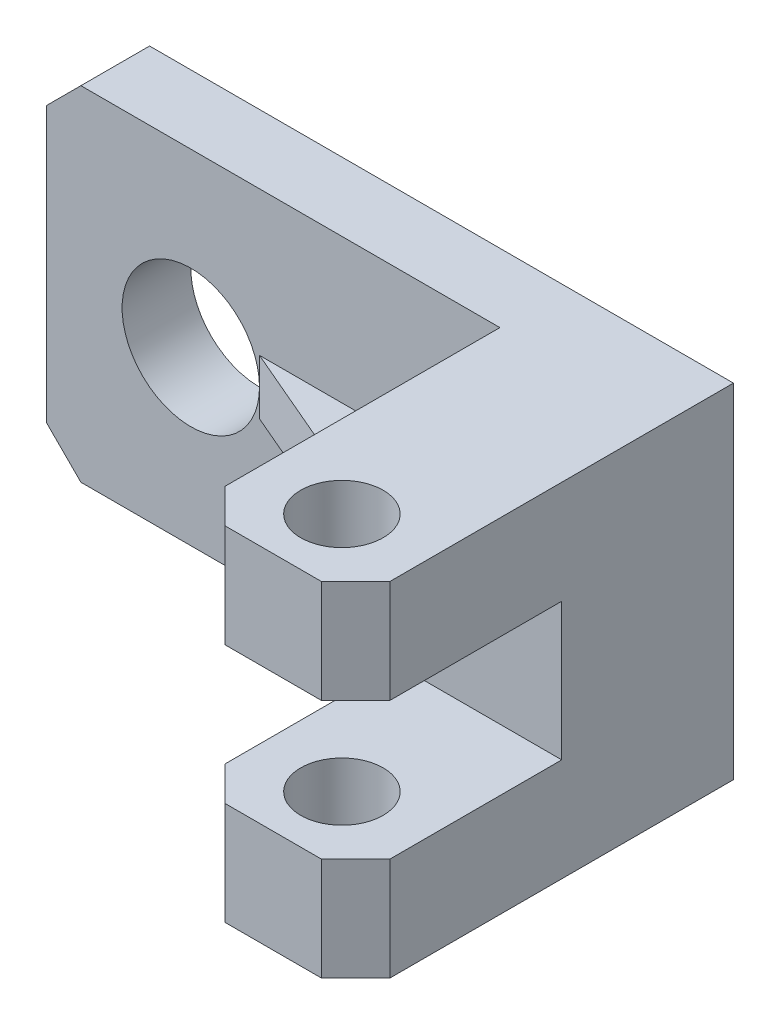
ISO-10303-21;
HEADER;
FILE_DESCRIPTION(('STEP AP214'),'2;1');
FILE_NAME('part.step','',(''),(''),'','','');
FILE_SCHEMA(('AUTOMOTIVE_DESIGN { 1 0 10303 214 1 1 1 1 }'));
ENDSEC;
DATA;
#1=APPLICATION_CONTEXT('core data for automotive mechanical design processes');
#2=APPLICATION_PROTOCOL_DEFINITION('international standard','automotive_design',2000,#1);
#3=PRODUCT_CONTEXT('',#1,'mechanical');
#4=PRODUCT('Part','Part','',(#3));
#5=PRODUCT_RELATED_PRODUCT_CATEGORY('part','',(#4));
#6=PRODUCT_DEFINITION_FORMATION('','',#4);
#7=PRODUCT_DEFINITION_CONTEXT('part definition',#1,'design');
#8=PRODUCT_DEFINITION('design','',#6,#7);
#9=PRODUCT_DEFINITION_SHAPE('','',#8);
#10=(LENGTH_UNIT() NAMED_UNIT(*) SI_UNIT(.MILLI.,.METRE.));
#11=(NAMED_UNIT(*) PLANE_ANGLE_UNIT() SI_UNIT($,.RADIAN.));
#12=(NAMED_UNIT(*) SI_UNIT($,.STERADIAN.) SOLID_ANGLE_UNIT());
#13=UNCERTAINTY_MEASURE_WITH_UNIT(LENGTH_MEASURE(1.E-05),#10,'distance_accuracy_value','');
#14=(GEOMETRIC_REPRESENTATION_CONTEXT(3) GLOBAL_UNCERTAINTY_ASSIGNED_CONTEXT((#13)) GLOBAL_UNIT_ASSIGNED_CONTEXT((#10,
#11,#12)) REPRESENTATION_CONTEXT('',''));
#15=CARTESIAN_POINT('',(0.,0.,0.));
#16=DIRECTION('',(0.,0.,1.));
#17=DIRECTION('',(1.,0.,0.));
#18=AXIS2_PLACEMENT_3D('',#15,#16,#17);
#19=CARTESIAN_POINT('',(66.,50.,50.));
#20=DIRECTION('',(-1.,0.,0.));
#21=DIRECTION('',(0.,0.,1.));
#22=AXIS2_PLACEMENT_3D('',#19,#20,#21);
#23=PLANE('',#22);
#24=DIRECTION('',(0.,-1.,0.));
#25=VECTOR('',#24,1.);
#26=CARTESIAN_POINT('',(66.,15.,25.));
#27=LINE('',#26,#25);
#28=CARTESIAN_POINT('',(66.,35.,25.));
#29=VERTEX_POINT('',#28);
#30=CARTESIAN_POINT('',(66.,29.,25.));
#31=VERTEX_POINT('',#30);
#32=EDGE_CURVE('E198',#29,#31,#27,.T.);
#33=ORIENTED_EDGE('',*,*,#32,.F.);
#34=DIRECTION('',(0.,0.,1.));
#35=VECTOR('',#34,1.);
#36=CARTESIAN_POINT('',(66.,35.,30.));
#37=LINE('',#36,#35);
#38=CARTESIAN_POINT('',(66.,35.,50.));
#39=VERTEX_POINT('',#38);
#40=EDGE_CURVE('E182',#29,#39,#37,.T.);
#41=ORIENTED_EDGE('',*,*,#40,.T.);
#42=DIRECTION('',(0.,-1.,0.));
#43=VECTOR('',#42,1.);
#44=CARTESIAN_POINT('',(66.,50.,50.));
#45=LINE('',#44,#43);
#46=CARTESIAN_POINT('',(66.,50.,50.));
#47=VERTEX_POINT('',#46);
#48=EDGE_CURVE('E290',#47,#39,#45,.T.);
#49=ORIENTED_EDGE('',*,*,#48,.F.);
#50=DIRECTION('',(0.,0.,-1.));
#51=VECTOR('',#50,1.);
#52=CARTESIAN_POINT('',(66.,50.,50.));
#53=LINE('',#52,#51);
#54=CARTESIAN_POINT('',(66.,50.,10.));
#55=VERTEX_POINT('',#54);
#56=EDGE_CURVE('E277',#47,#55,#53,.T.);
#57=ORIENTED_EDGE('',*,*,#56,.T.);
#58=DIRECTION('',(0.,1.,0.));
#59=VECTOR('',#58,1.);
#60=CARTESIAN_POINT('',(66.,29.,10.));
#61=LINE('',#60,#59);
#62=CARTESIAN_POINT('',(66.,29.,10.));
#63=VERTEX_POINT('',#62);
#64=EDGE_CURVE('E217',#63,#55,#61,.T.);
#65=ORIENTED_EDGE('',*,*,#64,.F.);
#66=DIRECTION('',(0.,0.,-1.));
#67=VECTOR('',#66,1.);
#68=CARTESIAN_POINT('',(66.,29.,25.));
#69=LINE('',#68,#67);
#70=EDGE_CURVE('E207',#31,#63,#69,.T.);
#71=ORIENTED_EDGE('',*,*,#70,.F.);
#72=EDGE_LOOP('',(#33,#41,#49,#57,#65,#71));
#73=FACE_BOUND('',#72,.T.);
#74=ADVANCED_FACE('F44',(#73),#23,.T.);
#75=CARTESIAN_POINT('',(31.,50.,10.));
#76=DIRECTION('',(-0.393919298579168,0.,0.919145030018058));
#77=DIRECTION('',(0.919145030018058,0.,0.393919298579168));
#78=AXIS2_PLACEMENT_3D('',#75,#76,#77);
#79=PLANE('',#78);
#80=DIRECTION('',(0.,-1.,0.));
#81=VECTOR('',#80,1.);
#82=CARTESIAN_POINT('',(66.,50.,25.));
#83=LINE('',#82,#81);
#84=CARTESIAN_POINT('',(66.,21.,25.));
#85=VERTEX_POINT('',#84);
#86=EDGE_CURVE('E235',#31,#85,#83,.T.);
#87=ORIENTED_EDGE('',*,*,#86,.F.);
#88=DIRECTION('',(0.919145030018058,0.,0.393919298579168));
#89=VECTOR('',#88,1.);
#90=CARTESIAN_POINT('',(31.,29.,10.));
#91=LINE('',#90,#89);
#92=CARTESIAN_POINT('',(31.,29.,10.));
#93=VERTEX_POINT('',#92);
#94=EDGE_CURVE('E214',#93,#31,#91,.T.);
#95=ORIENTED_EDGE('',*,*,#94,.F.);
#96=DIRECTION('',(0.,-1.,0.));
#97=VECTOR('',#96,1.);
#98=CARTESIAN_POINT('',(31.,50.,10.));
#99=LINE('',#98,#97);
#100=CARTESIAN_POINT('',(31.,25.,10.));
#101=VERTEX_POINT('',#100);
#102=EDGE_CURVE('E231',#93,#101,#99,.T.);
#103=ORIENTED_EDGE('',*,*,#102,.T.);
#104=CARTESIAN_POINT('',(31.,21.,10.));
#105=VERTEX_POINT('',#104);
#106=EDGE_CURVE('E236',#101,#105,#99,.T.);
#107=ORIENTED_EDGE('',*,*,#106,.T.);
#108=DIRECTION('',(-0.919145030018058,0.,-0.393919298579168));
#109=VECTOR('',#108,1.);
#110=CARTESIAN_POINT('',(31.,21.,10.));
#111=LINE('',#110,#109);
#112=EDGE_CURVE('E220',#85,#105,#111,.T.);
#113=ORIENTED_EDGE('',*,*,#112,.F.);
#114=EDGE_LOOP('',(#87,#95,#103,#107,#113));
#115=FACE_BOUND('',#114,.T.);
#116=ADVANCED_FACE('F365',(#115),#79,.T.);
#117=CARTESIAN_POINT('',(71.,50.,55.));
#118=DIRECTION('',(-0.707106781186547,0.,0.707106781186548));
#119=DIRECTION('',(0.707106781186548,0.,0.707106781186547));
#120=AXIS2_PLACEMENT_3D('',#117,#118,#119);
#121=PLANE('',#120);
#122=DIRECTION('',(-0.707106781186548,0.,-0.707106781186547));
#123=VECTOR('',#122,1.);
#124=CARTESIAN_POINT('',(71.,35.,55.));
#125=LINE('',#124,#123);
#126=CARTESIAN_POINT('',(71.,35.,55.));
#127=VERTEX_POINT('',#126);
#128=EDGE_CURVE('E188',#127,#39,#125,.T.);
#129=ORIENTED_EDGE('',*,*,#128,.F.);
#130=DIRECTION('',(0.,-1.,0.));
#131=VECTOR('',#130,1.);
#132=CARTESIAN_POINT('',(71.,50.,55.));
#133=LINE('',#132,#131);
#134=CARTESIAN_POINT('',(71.,50.,55.));
#135=VERTEX_POINT('',#134);
#136=EDGE_CURVE('E291',#135,#127,#133,.T.);
#137=ORIENTED_EDGE('',*,*,#136,.F.);
#138=DIRECTION('',(-0.707106781186548,0.,-0.707106781186547));
#139=VECTOR('',#138,1.);
#140=CARTESIAN_POINT('',(71.,50.,55.));
#141=LINE('',#140,#139);
#142=EDGE_CURVE('E271',#135,#47,#141,.T.);
#143=ORIENTED_EDGE('',*,*,#142,.T.);
#144=ORIENTED_EDGE('',*,*,#48,.T.);
#145=EDGE_LOOP('',(#129,#137,#143,#144));
#146=FACE_BOUND('',#145,.T.);
#147=ADVANCED_FACE('F368',(#146),#121,.T.);
#148=CARTESIAN_POINT('',(71.,50.,55.));
#149=DIRECTION('',(0.,0.,1.));
#150=DIRECTION('',(1.,0.,0.));
#151=AXIS2_PLACEMENT_3D('',#148,#149,#150);
#152=PLANE('',#151);
#153=DIRECTION('',(-1.,0.,0.));
#154=VECTOR('',#153,1.);
#155=CARTESIAN_POINT('',(66.,35.,55.));
#156=LINE('',#155,#154);
#157=CARTESIAN_POINT('',(85.,35.,55.));
#158=VERTEX_POINT('',#157);
#159=EDGE_CURVE('E242',#158,#127,#156,.T.);
#160=ORIENTED_EDGE('',*,*,#159,.F.);
#161=DIRECTION('',(0.,-1.,0.));
#162=VECTOR('',#161,1.);
#163=CARTESIAN_POINT('',(85.,50.,55.));
#164=LINE('',#163,#162);
#165=CARTESIAN_POINT('',(85.,50.,55.));
#166=VERTEX_POINT('',#165);
#167=EDGE_CURVE('E300',#166,#158,#164,.T.);
#168=ORIENTED_EDGE('',*,*,#167,.F.);
#169=DIRECTION('',(-1.,0.,0.));
#170=VECTOR('',#169,1.);
#171=CARTESIAN_POINT('',(71.,50.,55.));
#172=LINE('',#171,#170);
#173=EDGE_CURVE('E270',#166,#135,#172,.T.);
#174=ORIENTED_EDGE('',*,*,#173,.T.);
#175=ORIENTED_EDGE('',*,*,#136,.T.);
#176=EDGE_LOOP('',(#160,#168,#174,#175));
#177=FACE_BOUND('',#176,.T.);
#178=ADVANCED_FACE('F428',(#177),#152,.T.);
#179=CARTESIAN_POINT('',(85.,50.,55.));
#180=DIRECTION('',(0.707106781186547,0.,0.707106781186548));
#181=DIRECTION('',(0.707106781186548,0.,-0.707106781186547));
#182=AXIS2_PLACEMENT_3D('',#179,#180,#181);
#183=PLANE('',#182);
#184=DIRECTION('',(-0.707106781186548,0.,0.707106781186547));
#185=VECTOR('',#184,1.);
#186=CARTESIAN_POINT('',(85.,35.,55.));
#187=LINE('',#186,#185);
#188=CARTESIAN_POINT('',(90.,35.,50.));
#189=VERTEX_POINT('',#188);
#190=EDGE_CURVE('E257',#189,#158,#187,.T.);
#191=ORIENTED_EDGE('',*,*,#190,.F.);
#192=DIRECTION('',(0.,-1.,0.));
#193=VECTOR('',#192,1.);
#194=CARTESIAN_POINT('',(90.,50.,50.));
#195=LINE('',#194,#193);
#196=CARTESIAN_POINT('',(90.,50.,50.));
#197=VERTEX_POINT('',#196);
#198=EDGE_CURVE('E301',#197,#189,#195,.T.);
#199=ORIENTED_EDGE('',*,*,#198,.F.);
#200=DIRECTION('',(-0.707106781186548,0.,0.707106781186547));
#201=VECTOR('',#200,1.);
#202=CARTESIAN_POINT('',(85.,50.,55.));
#203=LINE('',#202,#201);
#204=EDGE_CURVE('E268',#197,#166,#203,.T.);
#205=ORIENTED_EDGE('',*,*,#204,.T.);
#206=ORIENTED_EDGE('',*,*,#167,.T.);
#207=EDGE_LOOP('',(#191,#199,#205,#206));
#208=FACE_BOUND('',#207,.T.);
#209=ADVANCED_FACE('F429',(#208),#183,.T.);
#210=CARTESIAN_POINT('',(78.,50.,45.));
#211=DIRECTION('',(0.,-1.,0.));
#212=DIRECTION('',(0.,0.,-1.));
#213=AXIS2_PLACEMENT_3D('',#210,#211,#212);
#214=CYLINDRICAL_SURFACE('',#213,6.);
#215=CARTESIAN_POINT('',(78.,35.,45.));
#216=DIRECTION('',(0.,1.,0.));
#217=DIRECTION('',(0.,0.,1.));
#218=AXIS2_PLACEMENT_3D('',#215,#216,#217);
#219=CIRCLE('',#218,6.);
#220=CARTESIAN_POINT('',(78.,35.,51.));
#221=VERTEX_POINT('',#220);
#222=EDGE_CURVE('E47',#221,#221,#219,.F.);
#223=ORIENTED_EDGE('',*,*,#222,.T.);
#224=EDGE_LOOP('',(#223));
#225=FACE_BOUND('',#224,.T.);
#226=CARTESIAN_POINT('',(78.,50.,45.));
#227=DIRECTION('',(0.,-1.,0.));
#228=DIRECTION('',(0.,0.,-1.));
#229=AXIS2_PLACEMENT_3D('',#226,#227,#228);
#230=CIRCLE('',#229,6.);
#231=CARTESIAN_POINT('',(78.,50.,39.));
#232=VERTEX_POINT('',#231);
#233=EDGE_CURVE('E258',#232,#232,#230,.T.);
#234=ORIENTED_EDGE('',*,*,#233,.F.);
#235=EDGE_LOOP('',(#234));
#236=FACE_BOUND('',#235,.T.);
#237=ADVANCED_FACE('F435',(#225,#236),#214,.F.);
#238=CARTESIAN_POINT('',(0.,0.,10.));
#239=DIRECTION('',(0.,0.,-1.));
#240=DIRECTION('',(-1.,0.,0.));
#241=AXIS2_PLACEMENT_3D('',#238,#239,#240);
#242=PLANE('',#241);
#243=DIRECTION('',(1.,0.,0.));
#244=VECTOR('',#243,1.);
#245=CARTESIAN_POINT('',(90.,0.,10.));
#246=LINE('',#245,#244);
#247=CARTESIAN_POINT('',(4.99999999999999,0.,10.));
#248=VERTEX_POINT('',#247);
#249=CARTESIAN_POINT('',(66.,0.,10.));
#250=VERTEX_POINT('',#249);
#251=EDGE_CURVE('E315',#248,#250,#246,.T.);
#252=ORIENTED_EDGE('',*,*,#251,.T.);
#253=DIRECTION('',(0.,-1.,0.));
#254=VECTOR('',#253,1.);
#255=CARTESIAN_POINT('',(66.,21.,10.));
#256=LINE('',#255,#254);
#257=CARTESIAN_POINT('',(66.,21.,10.));
#258=VERTEX_POINT('',#257);
#259=EDGE_CURVE('E230',#258,#250,#256,.T.);
#260=ORIENTED_EDGE('',*,*,#259,.F.);
#261=DIRECTION('',(1.,0.,0.));
#262=VECTOR('',#261,1.);
#263=CARTESIAN_POINT('',(66.,21.,10.));
#264=LINE('',#263,#262);
#265=EDGE_CURVE('E222',#105,#258,#264,.T.);
#266=ORIENTED_EDGE('',*,*,#265,.F.);
#267=ORIENTED_EDGE('',*,*,#106,.F.);
#268=CARTESIAN_POINT('',(21.,25.,10.));
#269=DIRECTION('',(0.,0.,1.));
#270=DIRECTION('',(1.,0.,0.));
#271=AXIS2_PLACEMENT_3D('',#268,#269,#270);
#272=CIRCLE('',#271,9.99999999999999);
#273=EDGE_CURVE('E232',#101,#101,#272,.T.);
#274=ORIENTED_EDGE('',*,*,#273,.F.);
#275=ORIENTED_EDGE('',*,*,#102,.F.);
#276=DIRECTION('',(-1.,0.,0.));
#277=VECTOR('',#276,1.);
#278=CARTESIAN_POINT('',(66.,29.,10.));
#279=LINE('',#278,#277);
#280=EDGE_CURVE('E65',#63,#93,#279,.T.);
#281=ORIENTED_EDGE('',*,*,#280,.F.);
#282=ORIENTED_EDGE('',*,*,#64,.T.);
#283=DIRECTION('',(-1.,0.,0.));
#284=VECTOR('',#283,1.);
#285=CARTESIAN_POINT('',(90.,50.,10.));
#286=LINE('',#285,#284);
#287=CARTESIAN_POINT('',(4.99999999999999,50.,10.));
#288=VERTEX_POINT('',#287);
#289=EDGE_CURVE('E314',#55,#288,#286,.T.);
#290=ORIENTED_EDGE('',*,*,#289,.T.);
#291=DIRECTION('',(-0.707106781186547,-0.707106781186548,0.));
#292=VECTOR('',#291,1.);
#293=CARTESIAN_POINT('',(0.,45.,10.));
#294=LINE('',#293,#292);
#295=CARTESIAN_POINT('',(0.,45.,10.));
#296=VERTEX_POINT('',#295);
#297=EDGE_CURVE('E302',#288,#296,#294,.T.);
#298=ORIENTED_EDGE('',*,*,#297,.T.);
#299=DIRECTION('',(0.,-1.,0.));
#300=VECTOR('',#299,1.);
#301=CARTESIAN_POINT('',(0.,45.,10.));
#302=LINE('',#301,#300);
#303=CARTESIAN_POINT('',(0.,5.,10.));
#304=VERTEX_POINT('',#303);
#305=EDGE_CURVE('E310',#296,#304,#302,.T.);
#306=ORIENTED_EDGE('',*,*,#305,.T.);
#307=DIRECTION('',(0.707106781186546,-0.707106781186548,0.));
#308=VECTOR('',#307,1.);
#309=CARTESIAN_POINT('',(0.,5.,10.));
#310=LINE('',#309,#308);
#311=EDGE_CURVE('E309',#304,#248,#310,.T.);
#312=ORIENTED_EDGE('',*,*,#311,.T.);
#313=EDGE_LOOP('',(#252,#260,#266,#267,#274,#275,#281,#282,#290,#298,#306,#312));
#314=FACE_BOUND('',#313,.T.);
#315=ADVANCED_FACE('F417',(#314),#242,.F.);
#316=CARTESIAN_POINT('',(0.,45.,10.));
#317=DIRECTION('',(0.707106781186548,-0.707106781186547,0.));
#318=DIRECTION('',(0.707106781186547,0.707106781186548,0.));
#319=AXIS2_PLACEMENT_3D('',#316,#317,#318);
#320=PLANE('',#319);
#321=DIRECTION('',(-0.707106781186547,-0.707106781186548,0.));
#322=VECTOR('',#321,1.);
#323=CARTESIAN_POINT('',(0.,45.,0.));
#324=LINE('',#323,#322);
#325=CARTESIAN_POINT('',(4.99999999999999,50.,0.));
#326=VERTEX_POINT('',#325);
#327=CARTESIAN_POINT('',(0.,45.,0.));
#328=VERTEX_POINT('',#327);
#329=EDGE_CURVE('E293',#326,#328,#324,.T.);
#330=ORIENTED_EDGE('',*,*,#329,.T.);
#331=DIRECTION('',(0.,0.,-1.));
#332=VECTOR('',#331,1.);
#333=CARTESIAN_POINT('',(0.,45.,10.));
#334=LINE('',#333,#332);
#335=EDGE_CURVE('E11',#296,#328,#334,.T.);
#336=ORIENTED_EDGE('',*,*,#335,.F.);
#337=ORIENTED_EDGE('',*,*,#297,.F.);
#338=DIRECTION('',(0.,0.,-1.));
#339=VECTOR('',#338,1.);
#340=CARTESIAN_POINT('',(4.99999999999999,50.,10.));
#341=LINE('',#340,#339);
#342=EDGE_CURVE('E320',#288,#326,#341,.T.);
#343=ORIENTED_EDGE('',*,*,#342,.T.);
#344=EDGE_LOOP('',(#330,#336,#337,#343));
#345=FACE_BOUND('',#344,.T.);
#346=ADVANCED_FACE('F50',(#345),#320,.F.);
#347=CARTESIAN_POINT('',(0.,45.,10.));
#348=DIRECTION('',(1.,0.,0.));
#349=DIRECTION('',(0.,0.,-1.));
#350=AXIS2_PLACEMENT_3D('',#347,#348,#349);
#351=PLANE('',#350);
#352=DIRECTION('',(0.,-1.,0.));
#353=VECTOR('',#352,1.);
#354=CARTESIAN_POINT('',(0.,45.,0.));
#355=LINE('',#354,#353);
#356=CARTESIAN_POINT('',(0.,5.,0.));
#357=VERTEX_POINT('',#356);
#358=EDGE_CURVE('E318',#328,#357,#355,.T.);
#359=ORIENTED_EDGE('',*,*,#358,.T.);
#360=DIRECTION('',(0.,0.,-1.));
#361=VECTOR('',#360,1.);
#362=CARTESIAN_POINT('',(0.,5.,10.));
#363=LINE('',#362,#361);
#364=EDGE_CURVE('E53',#304,#357,#363,.T.);
#365=ORIENTED_EDGE('',*,*,#364,.F.);
#366=ORIENTED_EDGE('',*,*,#305,.F.);
#367=ORIENTED_EDGE('',*,*,#335,.T.);
#368=EDGE_LOOP('',(#359,#365,#366,#367));
#369=FACE_BOUND('',#368,.T.);
#370=ADVANCED_FACE('F532',(#369),#351,.F.);
#371=CARTESIAN_POINT('',(0.,5.,10.));
#372=DIRECTION('',(0.707106781186548,0.707106781186546,0.));
#373=DIRECTION('',(-0.707106781186547,0.707106781186549,0.));
#374=AXIS2_PLACEMENT_3D('',#371,#372,#373);
#375=PLANE('',#374);
#376=DIRECTION('',(0.707106781186546,-0.707106781186548,0.));
#377=VECTOR('',#376,1.);
#378=CARTESIAN_POINT('',(0.,5.,0.));
#379=LINE('',#378,#377);
#380=CARTESIAN_POINT('',(4.99999999999999,0.,0.));
#381=VERTEX_POINT('',#380);
#382=EDGE_CURVE('E325',#357,#381,#379,.T.);
#383=ORIENTED_EDGE('',*,*,#382,.T.);
#384=DIRECTION('',(0.,0.,-1.));
#385=VECTOR('',#384,1.);
#386=CARTESIAN_POINT('',(4.99999999999999,0.,10.));
#387=LINE('',#386,#385);
#388=EDGE_CURVE('E340',#248,#381,#387,.T.);
#389=ORIENTED_EDGE('',*,*,#388,.F.);
#390=ORIENTED_EDGE('',*,*,#311,.F.);
#391=ORIENTED_EDGE('',*,*,#364,.T.);
#392=EDGE_LOOP('',(#383,#389,#390,#391));
#393=FACE_BOUND('',#392,.T.);
#394=ADVANCED_FACE('F518',(#393),#375,.F.);
#395=CARTESIAN_POINT('',(90.,0.,10.));
#396=DIRECTION('',(0.,1.,0.));
#397=DIRECTION('',(0.,0.,1.));
#398=AXIS2_PLACEMENT_3D('',#395,#396,#397);
#399=PLANE('',#398);
#400=CARTESIAN_POINT('',(78.,0.,45.));
#401=DIRECTION('',(0.,-1.,0.));
#402=DIRECTION('',(0.,0.,-1.));
#403=AXIS2_PLACEMENT_3D('',#400,#401,#402);
#404=CIRCLE('',#403,6.);
#405=CARTESIAN_POINT('',(78.,0.,39.));
#406=VERTEX_POINT('',#405);
#407=EDGE_CURVE('E256',#406,#406,#404,.T.);
#408=ORIENTED_EDGE('',*,*,#407,.F.);
#409=EDGE_LOOP('',(#408));
#410=FACE_BOUND('',#409,.T.);
#411=DIRECTION('',(0.,0.,-1.));
#412=VECTOR('',#411,1.);
#413=CARTESIAN_POINT('',(66.,0.,50.));
#414=LINE('',#413,#412);
#415=CARTESIAN_POINT('',(66.,0.,50.));
#416=VERTEX_POINT('',#415);
#417=EDGE_CURVE('E266',#416,#250,#414,.T.);
#418=ORIENTED_EDGE('',*,*,#417,.T.);
#419=ORIENTED_EDGE('',*,*,#251,.F.);
#420=ORIENTED_EDGE('',*,*,#388,.T.);
#421=DIRECTION('',(1.,0.,0.));
#422=VECTOR('',#421,1.);
#423=CARTESIAN_POINT('',(90.,0.,0.));
#424=LINE('',#423,#422);
#425=CARTESIAN_POINT('',(90.,0.,0.));
#426=VERTEX_POINT('',#425);
#427=EDGE_CURVE('E321',#381,#426,#424,.T.);
#428=ORIENTED_EDGE('',*,*,#427,.T.);
#429=DIRECTION('',(0.,0.,-1.));
#430=VECTOR('',#429,1.);
#431=CARTESIAN_POINT('',(90.,0.,10.));
#432=LINE('',#431,#430);
#433=CARTESIAN_POINT('',(90.,0.,50.));
#434=VERTEX_POINT('',#433);
#435=EDGE_CURVE('E335',#434,#426,#432,.T.);
#436=ORIENTED_EDGE('',*,*,#435,.F.);
#437=DIRECTION('',(-0.707106781186548,0.,0.707106781186547));
#438=VECTOR('',#437,1.);
#439=CARTESIAN_POINT('',(85.,0.,55.));
#440=LINE('',#439,#438);
#441=CARTESIAN_POINT('',(85.,0.,55.));
#442=VERTEX_POINT('',#441);
#443=EDGE_CURVE('E264',#434,#442,#440,.T.);
#444=ORIENTED_EDGE('',*,*,#443,.T.);
#445=DIRECTION('',(-1.,0.,0.));
#446=VECTOR('',#445,1.);
#447=CARTESIAN_POINT('',(71.,0.,55.));
#448=LINE('',#447,#446);
#449=CARTESIAN_POINT('',(71.,0.,55.));
#450=VERTEX_POINT('',#449);
#451=EDGE_CURVE('E282',#442,#450,#448,.T.);
#452=ORIENTED_EDGE('',*,*,#451,.T.);
#453=DIRECTION('',(-0.707106781186548,0.,-0.707106781186547));
#454=VECTOR('',#453,1.);
#455=CARTESIAN_POINT('',(71.,0.,55.));
#456=LINE('',#455,#454);
#457=EDGE_CURVE('E285',#450,#416,#456,.T.);
#458=ORIENTED_EDGE('',*,*,#457,.T.);
#459=EDGE_LOOP('',(#418,#419,#420,#428,#436,#444,#452,#458));
#460=FACE_BOUND('',#459,.T.);
#461=ADVANCED_FACE('F401',(#410,#460),#399,.F.);
#462=CARTESIAN_POINT('',(90.,0.,10.));
#463=DIRECTION('',(-1.,0.,0.));
#464=DIRECTION('',(0.,0.,1.));
#465=AXIS2_PLACEMENT_3D('',#462,#463,#464);
#466=PLANE('',#465);
#467=DIRECTION('',(0.,0.,1.));
#468=VECTOR('',#467,1.);
#469=CARTESIAN_POINT('',(90.,35.,30.));
#470=LINE('',#469,#468);
#471=CARTESIAN_POINT('',(90.,35.,25.));
#472=VERTEX_POINT('',#471);
#473=EDGE_CURVE('E193',#472,#189,#470,.T.);
#474=ORIENTED_EDGE('',*,*,#473,.F.);
#475=DIRECTION('',(0.,1.,0.));
#476=VECTOR('',#475,1.);
#477=CARTESIAN_POINT('',(90.,35.,25.));
#478=LINE('',#477,#476);
#479=CARTESIAN_POINT('',(90.,15.,25.));
#480=VERTEX_POINT('',#479);
#481=EDGE_CURVE('E202',#480,#472,#478,.T.);
#482=ORIENTED_EDGE('',*,*,#481,.F.);
#483=DIRECTION('',(0.,0.,1.));
#484=VECTOR('',#483,1.);
#485=CARTESIAN_POINT('',(90.,15.,30.));
#486=LINE('',#485,#484);
#487=CARTESIAN_POINT('',(90.,15.,50.));
#488=VERTEX_POINT('',#487);
#489=EDGE_CURVE('E247',#480,#488,#486,.T.);
#490=ORIENTED_EDGE('',*,*,#489,.T.);
#491=EDGE_CURVE('E276',#488,#434,#195,.T.);
#492=ORIENTED_EDGE('',*,*,#491,.T.);
#493=ORIENTED_EDGE('',*,*,#435,.T.);
#494=DIRECTION('',(0.,1.,0.));
#495=VECTOR('',#494,1.);
#496=CARTESIAN_POINT('',(90.,0.,0.));
#497=LINE('',#496,#495);
#498=CARTESIAN_POINT('',(90.,50.,0.));
#499=VERTEX_POINT('',#498);
#500=EDGE_CURVE('E326',#426,#499,#497,.T.);
#501=ORIENTED_EDGE('',*,*,#500,.T.);
#502=DIRECTION('',(0.,0.,-1.));
#503=VECTOR('',#502,1.);
#504=CARTESIAN_POINT('',(90.,50.,10.));
#505=LINE('',#504,#503);
#506=EDGE_CURVE('E333',#197,#499,#505,.T.);
#507=ORIENTED_EDGE('',*,*,#506,.F.);
#508=ORIENTED_EDGE('',*,*,#198,.T.);
#509=EDGE_LOOP('',(#474,#482,#490,#492,#493,#501,#507,#508));
#510=FACE_BOUND('',#509,.T.);
#511=ADVANCED_FACE('F395',(#510),#466,.F.);
#512=CARTESIAN_POINT('',(90.,50.,10.));
#513=DIRECTION('',(0.,-1.,0.));
#514=DIRECTION('',(0.,0.,-1.));
#515=AXIS2_PLACEMENT_3D('',#512,#513,#514);
#516=PLANE('',#515);
#517=ORIENTED_EDGE('',*,*,#289,.F.);
#518=ORIENTED_EDGE('',*,*,#56,.F.);
#519=ORIENTED_EDGE('',*,*,#142,.F.);
#520=ORIENTED_EDGE('',*,*,#173,.F.);
#521=ORIENTED_EDGE('',*,*,#204,.F.);
#522=ORIENTED_EDGE('',*,*,#506,.T.);
#523=DIRECTION('',(-1.,0.,0.));
#524=VECTOR('',#523,1.);
#525=CARTESIAN_POINT('',(90.,50.,0.));
#526=LINE('',#525,#524);
#527=EDGE_CURVE('E308',#499,#326,#526,.T.);
#528=ORIENTED_EDGE('',*,*,#527,.T.);
#529=ORIENTED_EDGE('',*,*,#342,.F.);
#530=EDGE_LOOP('',(#517,#518,#519,#520,#521,#522,#528,#529));
#531=FACE_BOUND('',#530,.T.);
#532=ORIENTED_EDGE('',*,*,#233,.T.);
#533=EDGE_LOOP('',(#532));
#534=FACE_BOUND('',#533,.T.);
#535=ADVANCED_FACE('F384',(#531,#534),#516,.F.);
#536=CARTESIAN_POINT('',(0.,0.,0.));
#537=DIRECTION('',(0.,0.,-1.));
#538=DIRECTION('',(-1.,0.,0.));
#539=AXIS2_PLACEMENT_3D('',#536,#537,#538);
#540=PLANE('',#539);
#541=CARTESIAN_POINT('',(21.,25.,0.));
#542=DIRECTION('',(0.,0.,1.));
#543=DIRECTION('',(1.,0.,0.));
#544=AXIS2_PLACEMENT_3D('',#541,#542,#543);
#545=CIRCLE('',#544,9.99999999999999);
#546=CARTESIAN_POINT('',(31.,25.,0.));
#547=VERTEX_POINT('',#546);
#548=EDGE_CURVE('E238',#547,#547,#545,.T.);
#549=ORIENTED_EDGE('',*,*,#548,.T.);
#550=EDGE_LOOP('',(#549));
#551=FACE_BOUND('',#550,.T.);
#552=ORIENTED_EDGE('',*,*,#329,.F.);
#553=ORIENTED_EDGE('',*,*,#527,.F.);
#554=ORIENTED_EDGE('',*,*,#500,.F.);
#555=ORIENTED_EDGE('',*,*,#427,.F.);
#556=ORIENTED_EDGE('',*,*,#382,.F.);
#557=ORIENTED_EDGE('',*,*,#358,.F.);
#558=EDGE_LOOP('',(#552,#553,#554,#555,#556,#557));
#559=FACE_BOUND('',#558,.T.);
#560=ADVANCED_FACE('F372',(#551,#559),#540,.T.);
#561=DIRECTION('',(0.,0.,1.));
#562=VECTOR('',#561,1.);
#563=CARTESIAN_POINT('',(66.,15.,30.));
#564=LINE('',#563,#562);
#565=CARTESIAN_POINT('',(66.,15.,25.));
#566=VERTEX_POINT('',#565);
#567=CARTESIAN_POINT('',(66.,15.,50.));
#568=VERTEX_POINT('',#567);
#569=EDGE_CURVE('E244',#566,#568,#564,.T.);
#570=ORIENTED_EDGE('',*,*,#569,.F.);
#571=EDGE_CURVE('E205',#85,#566,#27,.T.);
#572=ORIENTED_EDGE('',*,*,#571,.F.);
#573=DIRECTION('',(0.,0.,1.));
#574=VECTOR('',#573,1.);
#575=CARTESIAN_POINT('',(66.,21.,25.));
#576=LINE('',#575,#574);
#577=EDGE_CURVE('E228',#258,#85,#576,.T.);
#578=ORIENTED_EDGE('',*,*,#577,.F.);
#579=ORIENTED_EDGE('',*,*,#259,.T.);
#580=ORIENTED_EDGE('',*,*,#417,.F.);
#581=EDGE_CURVE('E292',#568,#416,#45,.T.);
#582=ORIENTED_EDGE('',*,*,#581,.F.);
#583=EDGE_LOOP('',(#570,#572,#578,#579,#580,#582));
#584=FACE_BOUND('',#583,.T.);
#585=ADVANCED_FACE('F364',(#584),#23,.T.);
#586=DIRECTION('',(0.707106781186548,0.,0.707106781186547));
#587=VECTOR('',#586,1.);
#588=CARTESIAN_POINT('',(71.,15.,55.));
#589=LINE('',#588,#587);
#590=CARTESIAN_POINT('',(71.,15.,55.));
#591=VERTEX_POINT('',#590);
#592=EDGE_CURVE('E251',#568,#591,#589,.T.);
#593=ORIENTED_EDGE('',*,*,#592,.F.);
#594=ORIENTED_EDGE('',*,*,#581,.T.);
#595=ORIENTED_EDGE('',*,*,#457,.F.);
#596=EDGE_CURVE('E298',#591,#450,#133,.T.);
#597=ORIENTED_EDGE('',*,*,#596,.F.);
#598=EDGE_LOOP('',(#593,#594,#595,#597));
#599=FACE_BOUND('',#598,.T.);
#600=ADVANCED_FACE('F373',(#599),#121,.T.);
#601=DIRECTION('',(1.,0.,0.));
#602=VECTOR('',#601,1.);
#603=CARTESIAN_POINT('',(66.,15.,55.));
#604=LINE('',#603,#602);
#605=CARTESIAN_POINT('',(85.,15.,55.));
#606=VERTEX_POINT('',#605);
#607=EDGE_CURVE('E70',#591,#606,#604,.T.);
#608=ORIENTED_EDGE('',*,*,#607,.F.);
#609=ORIENTED_EDGE('',*,*,#596,.T.);
#610=ORIENTED_EDGE('',*,*,#451,.F.);
#611=EDGE_CURVE('E297',#606,#442,#164,.T.);
#612=ORIENTED_EDGE('',*,*,#611,.F.);
#613=EDGE_LOOP('',(#608,#609,#610,#612));
#614=FACE_BOUND('',#613,.T.);
#615=ADVANCED_FACE('F379',(#614),#152,.T.);
#616=DIRECTION('',(0.707106781186548,0.,-0.707106781186547));
#617=VECTOR('',#616,1.);
#618=CARTESIAN_POINT('',(85.,15.,55.));
#619=LINE('',#618,#617);
#620=EDGE_CURVE('E255',#606,#488,#619,.T.);
#621=ORIENTED_EDGE('',*,*,#620,.F.);
#622=ORIENTED_EDGE('',*,*,#611,.T.);
#623=ORIENTED_EDGE('',*,*,#443,.F.);
#624=ORIENTED_EDGE('',*,*,#491,.F.);
#625=EDGE_LOOP('',(#621,#622,#623,#624));
#626=FACE_BOUND('',#625,.T.);
#627=ADVANCED_FACE('F400',(#626),#183,.T.);
#628=CARTESIAN_POINT('',(78.,15.,45.));
#629=DIRECTION('',(0.,-1.,0.));
#630=DIRECTION('',(0.,0.,-1.));
#631=AXIS2_PLACEMENT_3D('',#628,#629,#630);
#632=CIRCLE('',#631,6.);
#633=CARTESIAN_POINT('',(78.,15.,39.));
#634=VERTEX_POINT('',#633);
#635=EDGE_CURVE('E191',#634,#634,#632,.F.);
#636=ORIENTED_EDGE('',*,*,#635,.T.);
#637=EDGE_LOOP('',(#636));
#638=FACE_BOUND('',#637,.T.);
#639=ORIENTED_EDGE('',*,*,#407,.T.);
#640=EDGE_LOOP('',(#639));
#641=FACE_BOUND('',#640,.T.);
#642=ADVANCED_FACE('F341',(#638,#641),#214,.F.);
#643=CARTESIAN_POINT('',(66.,35.,30.));
#644=DIRECTION('',(0.,1.,0.));
#645=DIRECTION('',(0.,0.,1.));
#646=AXIS2_PLACEMENT_3D('',#643,#644,#645);
#647=PLANE('',#646);
#648=ORIENTED_EDGE('',*,*,#128,.T.);
#649=ORIENTED_EDGE('',*,*,#40,.F.);
#650=DIRECTION('',(-1.,0.,0.));
#651=VECTOR('',#650,1.);
#652=CARTESIAN_POINT('',(66.,35.,25.));
#653=LINE('',#652,#651);
#654=EDGE_CURVE('E190',#472,#29,#653,.T.);
#655=ORIENTED_EDGE('',*,*,#654,.F.);
#656=ORIENTED_EDGE('',*,*,#473,.T.);
#657=ORIENTED_EDGE('',*,*,#190,.T.);
#658=ORIENTED_EDGE('',*,*,#159,.T.);
#659=EDGE_LOOP('',(#648,#649,#655,#656,#657,#658));
#660=FACE_BOUND('',#659,.T.);
#661=ORIENTED_EDGE('',*,*,#222,.F.);
#662=EDGE_LOOP('',(#661));
#663=FACE_BOUND('',#662,.T.);
#664=ADVANCED_FACE('F184',(#660,#663),#647,.F.);
#665=CARTESIAN_POINT('',(66.,15.,30.));
#666=DIRECTION('',(0.,-1.,0.));
#667=DIRECTION('',(0.,0.,-1.));
#668=AXIS2_PLACEMENT_3D('',#665,#666,#667);
#669=PLANE('',#668);
#670=ORIENTED_EDGE('',*,*,#592,.T.);
#671=ORIENTED_EDGE('',*,*,#607,.T.);
#672=ORIENTED_EDGE('',*,*,#620,.T.);
#673=ORIENTED_EDGE('',*,*,#489,.F.);
#674=DIRECTION('',(1.,0.,0.));
#675=VECTOR('',#674,1.);
#676=CARTESIAN_POINT('',(90.,15.,25.));
#677=LINE('',#676,#675);
#678=EDGE_CURVE('E210',#566,#480,#677,.T.);
#679=ORIENTED_EDGE('',*,*,#678,.F.);
#680=ORIENTED_EDGE('',*,*,#569,.T.);
#681=EDGE_LOOP('',(#670,#671,#672,#673,#679,#680));
#682=FACE_BOUND('',#681,.T.);
#683=ORIENTED_EDGE('',*,*,#635,.F.);
#684=EDGE_LOOP('',(#683));
#685=FACE_BOUND('',#684,.T.);
#686=ADVANCED_FACE('F347',(#682,#685),#669,.F.);
#687=CARTESIAN_POINT('',(21.,25.,0.));
#688=DIRECTION('',(0.,0.,1.));
#689=DIRECTION('',(1.,0.,0.));
#690=AXIS2_PLACEMENT_3D('',#687,#688,#689);
#691=CYLINDRICAL_SURFACE('',#690,9.99999999999999);
#692=ORIENTED_EDGE('',*,*,#548,.F.);
#693=EDGE_LOOP('',(#692));
#694=FACE_BOUND('',#693,.T.);
#695=ORIENTED_EDGE('',*,*,#273,.T.);
#696=EDGE_LOOP('',(#695));
#697=FACE_BOUND('',#696,.T.);
#698=ADVANCED_FACE('F348',(#694,#697),#691,.F.);
#699=CARTESIAN_POINT('',(0.,21.,0.));
#700=DIRECTION('',(0.,1.,0.));
#701=DIRECTION('',(0.,0.,1.));
#702=AXIS2_PLACEMENT_3D('',#699,#700,#701);
#703=PLANE('',#702);
#704=ORIENTED_EDGE('',*,*,#112,.T.);
#705=ORIENTED_EDGE('',*,*,#265,.T.);
#706=ORIENTED_EDGE('',*,*,#577,.T.);
#707=EDGE_LOOP('',(#704,#705,#706));
#708=FACE_BOUND('',#707,.T.);
#709=ADVANCED_FACE('F358',(#708),#703,.F.);
#710=CARTESIAN_POINT('',(0.,29.,0.));
#711=DIRECTION('',(0.,1.,0.));
#712=DIRECTION('',(0.,0.,1.));
#713=AXIS2_PLACEMENT_3D('',#710,#711,#712);
#714=PLANE('',#713);
#715=ORIENTED_EDGE('',*,*,#94,.T.);
#716=ORIENTED_EDGE('',*,*,#70,.T.);
#717=ORIENTED_EDGE('',*,*,#280,.T.);
#718=EDGE_LOOP('',(#715,#716,#717));
#719=FACE_BOUND('',#718,.T.);
#720=ADVANCED_FACE('F458',(#719),#714,.T.);
#721=CARTESIAN_POINT('',(0.,0.,25.));
#722=DIRECTION('',(0.,0.,-1.));
#723=DIRECTION('',(-1.,0.,0.));
#724=AXIS2_PLACEMENT_3D('',#721,#722,#723);
#725=PLANE('',#724);
#726=ORIENTED_EDGE('',*,*,#654,.T.);
#727=ORIENTED_EDGE('',*,*,#32,.T.);
#728=ORIENTED_EDGE('',*,*,#86,.T.);
#729=ORIENTED_EDGE('',*,*,#571,.T.);
#730=ORIENTED_EDGE('',*,*,#678,.T.);
#731=ORIENTED_EDGE('',*,*,#481,.T.);
#732=EDGE_LOOP('',(#726,#727,#728,#729,#730,#731));
#733=FACE_BOUND('',#732,.T.);
#734=ADVANCED_FACE('F199',(#733),#725,.F.);
#735=CLOSED_SHELL('',(#74,#116,#147,#178,#209,#237,#315,#346,#370,#394,#461,#511,#535,#560,#585,
#600,#615,#627,#642,#664,#686,#698,#709,#720,#734));
#736=MANIFOLD_SOLID_BREP('B2',#735);
#737=ADVANCED_BREP_SHAPE_REPRESENTATION('',(#18,#736),#14);
#738=SHAPE_DEFINITION_REPRESENTATION(#9,#737);
ENDSEC;
END-ISO-10303-21;
